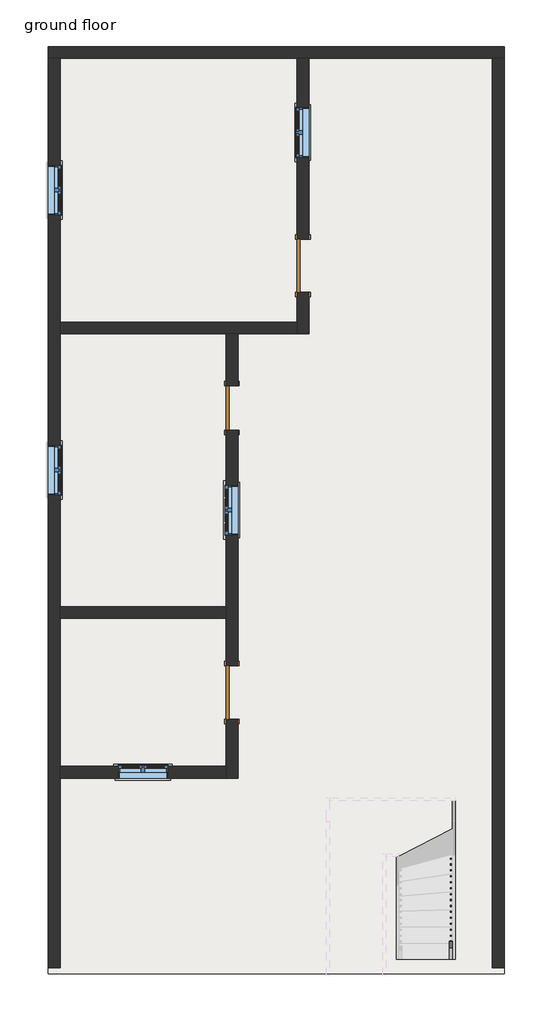
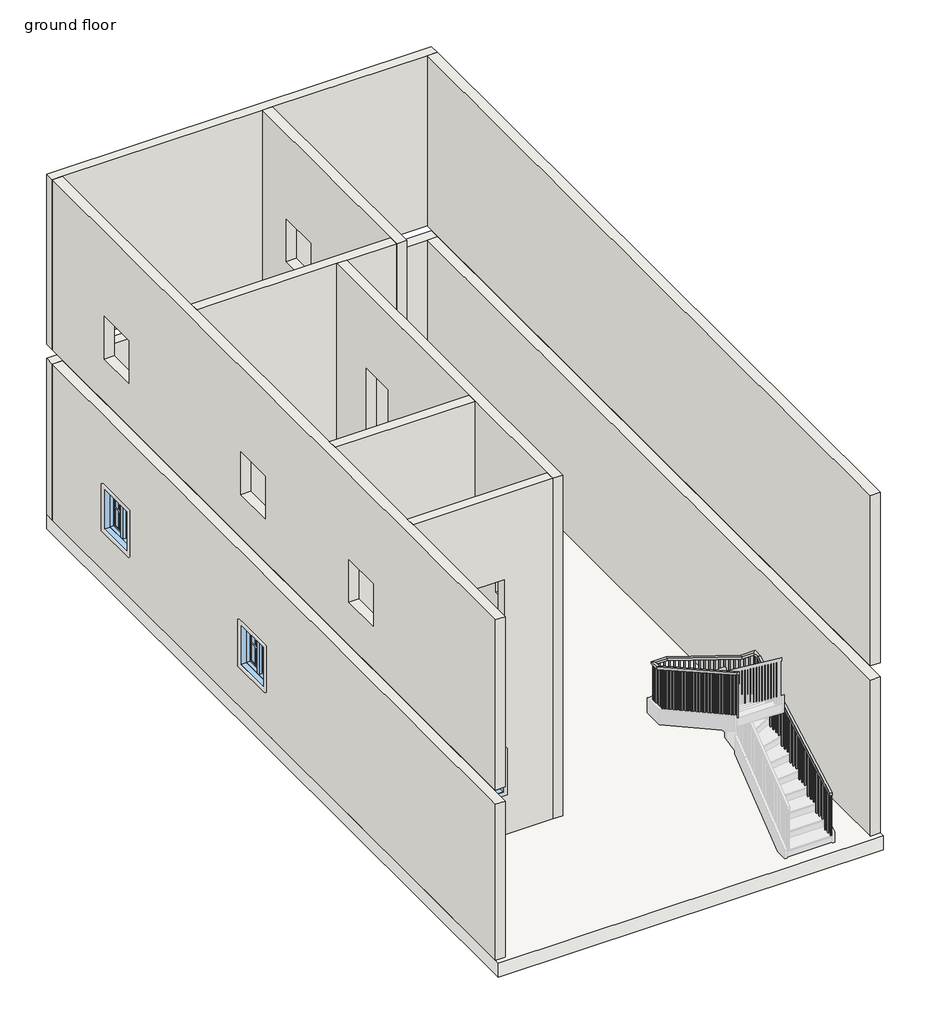
# One storey, part 1 of 2: 8 walls, 5 windows, 3 doors, 2 slabs, 1 railing.
"""IFC4 building model written with IfcOpenShell, lengths in millimetres."""

from ifc_helpers import new_model, si_unit, frame, origin, place, context, project, spatial, polyline, outline, extrude, faceted_brep, transform, mapped, element, save
from components import door_b6acaa4e, door_54dd4da4, door_719f80de, window_c29befe5, window_99681c7d

model = new_model("IFC4")

# Units and contexts
model_context = context("Model", 3, world=origin())
ifc_project = project(units=[si_unit("LENGTHUNIT", "METRE", prefix="MILLI")], contexts=[model_context])

# Site, building, storey
site = spatial("IfcSite", under=ifc_project)
building = spatial("IfcBuilding", under=site)
storey = spatial("IfcBuildingStorey", under=building, Name="ground floor", Elevation=1828.8)

# Doors
placement = place(None, origin())
door_shape = door_b6acaa4e(model_context)
element("IfcDoor", 1, ObjectType="Single-Flush : 30\" x 84\"", at=placement, inside=storey, context=model_context, shape_type="MappedRepresentation", body=[
    mapped(door_shape, transform((-12734.4887549, 9866.3027962, 1828.8), x_axis=(0.0, 1.0, 0.0), y_axis=(-1.0, 0.0, 0.0), z_axis=(0.0, 0.0, 1.0))),
])
door_2_shape = door_54dd4da4(model_context)
element("IfcDoor", 2, ObjectType="Single-Flush : 36\" x 84\"", at=placement, inside=storey, context=model_context, shape_type="MappedRepresentation", body=[
    mapped(door_2_shape, transform((-12734.4887549, 4989.5027962, 1828.8), x_axis=(0.0, 1.0, 0.0), y_axis=(-1.0, 0.0, 0.0), z_axis=(0.0, 0.0, 1.0))),
])
door_3_shape = door_719f80de(model_context)
element("IfcDoor", 3, ObjectType="Single-Flush : 36\" x 84\"", at=placement, inside=storey, context=model_context, shape_type="MappedRepresentation", body=[
    mapped(door_3_shape, transform((-11515.2887549, 12304.7027962, 1828.8), x_axis=(0.0, -1.0, 0.0), y_axis=(1.0, 0.0, 0.0), z_axis=(0.0, 0.0, 1.0))),
])

# Railing
element("IfcRailing", 4, ObjectType="Handrail - Rectangular", at=placement, inside=storey, context=model_context, shape_type="SolidModel", body=[
    faceted_brep([(-9000.6887549, 413.7711043, 2917.3714286), (-9000.6887549, 413.7711043, 2859.302637), (-8949.8887549, 413.7711043, 2859.302637), (-8949.8887549, 413.7711043, 2917.3714286), (-9000.6887549, 2949.2841703, 4321.4291136), (-9000.6887549, 2962.4104944, 4270.6291136), (-8949.8887549, 2962.4104944, 4270.6291136), (-8949.8887549, 2949.2841703, 4321.4291136), (-9252.9468652, 3084.5027962, 4270.6291136), (-9244.780431, 3084.5027962, 4321.4291136), (-10757.3244342, 3084.5027962, 4820.6326651), (-10765.4908683, 3084.5027962, 4769.8326651), (-9252.9468652, 3135.3027962, 4270.6291136), (-10765.4908683, 3135.3027962, 4769.8326651), (-9244.780431, 3135.3027962, 4321.4291136), (-10757.3244342, 3135.3027962, 4820.6326651), (-11007.2887549, 134.3711043, 6400.8), (-11058.0887549, 134.3711043, 6400.8), (-11058.0887549, 134.3711043, 6342.5372273), (-11007.2887549, 134.3711043, 6342.5372273), (-11007.2887549, 2934.7866859, 4769.8326651), (-11007.2887549, 2948.0751733, 4820.6326651), (-11058.0887549, 2934.7866859, 4769.8326651), (-11058.0887549, 2948.0751733, 4820.6326651), (-9000.6887549, 3084.5027962, 4321.4291136), (-9000.6887549, 3084.5027962, 4270.6291136), (-8949.8887549, 3135.3027962, 4270.6291136), (-8949.8887549, 3135.3027962, 4321.4291136), (-11007.2887549, 3084.5027962, 4820.6326651), (-11007.2887549, 3084.5027962, 4769.8326651), (-11058.0887549, 3135.3027962, 4769.8326651), (-11058.0887549, 3135.3027962, 4820.6326651)], [[[0, 1, 2, 3]], [[1, 0, 4, 5]], [[2, 1, 5, 6]], [[3, 2, 6, 7]], [[0, 3, 7, 4]], [[8, 9, 10, 11]], [[12, 8, 11, 13]], [[14, 12, 13, 15]], [[9, 14, 15, 10]], [[16, 17, 18, 19]], [[20, 21, 16, 19]], [[22, 20, 19, 18]], [[23, 22, 18, 17]], [[21, 23, 17, 16]], [[5, 4, 24, 25]], [[6, 5, 25, 26]], [[7, 6, 26, 27]], [[4, 7, 27, 24]], [[25, 24, 9, 8]], [[26, 25, 8, 12]], [[27, 26, 12, 14]], [[24, 27, 14, 9]], [[11, 10, 28, 29]], [[13, 11, 29, 30]], [[15, 13, 30, 31]], [[10, 15, 31, 28]], [[29, 28, 21, 20]], [[30, 29, 20, 22]], [[31, 30, 22, 23]], [[28, 31, 23, 21]]]),
    extrude(outline(polyline([(153.9777962, 6331.526171), (173.0277962, 6320.827751), (173.0277962, 5312.2285714), (153.9777962, 5312.2285714), (153.9777962, 6331.526171)])), frame((-11042.2137549, 0.0, 0.0), z_axis=(1.0, 0.0, 0.0), x_axis=(0.0, 1.0, 0.0)), (0.0, 0.0, 1.0), 19.05),
    extrude(outline(polyline([(255.5777962, 6274.4679313), (274.6277962, 6263.7695113), (274.6277962, 5312.2285714), (255.5777962, 5312.2285714), (255.5777962, 6274.4679313)])), frame((-11042.2137549, 0.0, 0.0), z_axis=(1.0, 0.0, 0.0), x_axis=(0.0, 1.0, 0.0)), (0.0, 0.0, 1.0), 19.05),
    extrude(outline(polyline([(357.1777962, 6217.4096916), (376.2277962, 6206.7112716), (376.2277962, 5312.2285714), (357.1777962, 5312.2285714), (357.1777962, 6217.4096916)])), frame((-11042.2137549, 0.0, 0.0), z_axis=(1.0, 0.0, 0.0), x_axis=(0.0, 1.0, 0.0)), (0.0, 0.0, 1.0), 19.05),
    extrude(outline(polyline([(458.7777962, 6160.3514519), (477.8277962, 6149.6530319), (477.8277962, 5138.0571429), (458.7777962, 5138.0571429), (458.7777962, 6160.3514519)])), frame((-11042.2137549, 0.0, 0.0), z_axis=(1.0, 0.0, 0.0), x_axis=(0.0, 1.0, 0.0)), (0.0, 0.0, 1.0), 19.05),
    extrude(outline(polyline([(560.3777962, 6103.2932122), (579.4277962, 6092.5947922), (579.4277962, 5138.0571429), (560.3777962, 5138.0571429), (560.3777962, 6103.2932122)])), frame((-11042.2137549, 0.0, 0.0), z_axis=(1.0, 0.0, 0.0), x_axis=(0.0, 1.0, 0.0)), (0.0, 0.0, 1.0), 19.05),
    extrude(outline(polyline([(661.9777962, 6046.2349725), (681.0277962, 6035.5365525), (681.0277962, 5138.0571429), (661.9777962, 5138.0571429), (661.9777962, 6046.2349725)])), frame((-11042.2137549, 0.0, 0.0), z_axis=(1.0, 0.0, 0.0), x_axis=(0.0, 1.0, 0.0)), (0.0, 0.0, 1.0), 19.05),
    extrude(outline(polyline([(763.5777962, 5989.1767328), (782.6277962, 5978.4783128), (782.6277962, 4963.8857143), (763.5777962, 4963.8857143), (763.5777962, 5989.1767328)])), frame((-11042.2137549, 0.0, 0.0), z_axis=(1.0, 0.0, 0.0), x_axis=(0.0, 1.0, 0.0)), (0.0, 0.0, 1.0), 19.05),
    extrude(outline(polyline([(865.1777962, 5932.1184931), (884.2277962, 5921.4200731), (884.2277962, 4963.8857143), (865.1777962, 4963.8857143), (865.1777962, 5932.1184931)])), frame((-11042.2137549, 0.0, 0.0), z_axis=(1.0, 0.0, 0.0), x_axis=(0.0, 1.0, 0.0)), (0.0, 0.0, 1.0), 19.05),
    extrude(outline(polyline([(966.7777962, 5875.0602534), (985.8277962, 5864.3618334), (985.8277962, 4963.8857143), (966.7777962, 4963.8857143), (966.7777962, 5875.0602534)])), frame((-11042.2137549, 0.0, 0.0), z_axis=(1.0, 0.0, 0.0), x_axis=(0.0, 1.0, 0.0)), (0.0, 0.0, 1.0), 19.05),
    extrude(outline(polyline([(1068.3777962, 5818.0020137), (1087.4277962, 5807.3035937), (1087.4277962, 4789.7142857), (1068.3777962, 4789.7142857), (1068.3777962, 5818.0020137)])), frame((-11042.2137549, 0.0, 0.0), z_axis=(1.0, 0.0, 0.0), x_axis=(0.0, 1.0, 0.0)), (0.0, 0.0, 1.0), 19.05),
    extrude(outline(polyline([(1169.9777962, 5760.943774), (1189.0277962, 5750.245354), (1189.0277962, 4789.7142857), (1169.9777962, 4789.7142857), (1169.9777962, 5760.943774)])), frame((-11042.2137549, 0.0, 0.0), z_axis=(1.0, 0.0, 0.0), x_axis=(0.0, 1.0, 0.0)), (0.0, 0.0, 1.0), 19.05),
    extrude(outline(polyline([(1271.5777962, 5703.8855343), (1290.6277962, 5693.1871143), (1290.6277962, 4615.5428571), (1271.5777962, 4615.5428571), (1271.5777962, 5703.8855343)])), frame((-11042.2137549, 0.0, 0.0), z_axis=(1.0, 0.0, 0.0), x_axis=(0.0, 1.0, 0.0)), (0.0, 0.0, 1.0), 19.05),
    extrude(outline(polyline([(1373.1777962, 5646.8272946), (1392.2277962, 5636.1288746), (1392.2277962, 4615.5428571), (1373.1777962, 4615.5428571), (1373.1777962, 5646.8272946)])), frame((-11042.2137549, 0.0, 0.0), z_axis=(1.0, 0.0, 0.0), x_axis=(0.0, 1.0, 0.0)), (0.0, 0.0, 1.0), 19.05),
    extrude(outline(polyline([(1474.7777962, 5589.6719878), (1493.8277962, 5579.1229201), (1493.8277962, 4615.5428571), (1474.7777962, 4615.5428571), (1474.7777962, 5589.6719878)])), frame((-11042.2137549, 0.0, 0.0), z_axis=(1.0, 0.0, 0.0), x_axis=(0.0, 1.0, 0.0)), (0.0, 0.0, 1.0), 19.05),
    extrude(outline(polyline([(1576.3777962, 5532.7108152), (1595.4277962, 5522.0123952), (1595.4277962, 4441.3714286), (1576.3777962, 4441.3714286), (1576.3777962, 5532.7108152)])), frame((-11042.2137549, 0.0, 0.0), z_axis=(1.0, 0.0, 0.0), x_axis=(0.0, 1.0, 0.0)), (0.0, 0.0, 1.0), 19.05),
    extrude(outline(polyline([(1677.9777962, 5475.6525755), (1697.0277962, 5464.9541555), (1697.0277962, 4441.3714286), (1677.9777962, 4441.3714286), (1677.9777962, 5475.6525755)])), frame((-11042.2137549, 0.0, 0.0), z_axis=(1.0, 0.0, 0.0), x_axis=(0.0, 1.0, 0.0)), (0.0, 0.0, 1.0), 19.05),
    extrude(outline(polyline([(1779.5777962, 5418.5943358), (1798.6277962, 5407.8959158), (1798.6277962, 4441.3714286), (1779.5777962, 4441.3714286), (1779.5777962, 5418.5943358)])), frame((-11042.2137549, 0.0, 0.0), z_axis=(1.0, 0.0, 0.0), x_axis=(0.0, 1.0, 0.0)), (0.0, 0.0, 1.0), 19.05),
    extrude(outline(polyline([(1881.1777962, 5361.536096), (1900.2277962, 5350.8376761), (1900.2277962, 4267.2), (1881.1777962, 4267.2), (1881.1777962, 5361.536096)])), frame((-11042.2137549, 0.0, 0.0), z_axis=(1.0, 0.0, 0.0), x_axis=(0.0, 1.0, 0.0)), (0.0, 0.0, 1.0), 19.05),
    extrude(outline(polyline([(1982.7777962, 5304.4778563), (2001.8277962, 5293.7794364), (2001.8277962, 4267.2), (1982.7777962, 4267.2), (1982.7777962, 5304.4778563)])), frame((-11042.2137549, 0.0, 0.0), z_axis=(1.0, 0.0, 0.0), x_axis=(0.0, 1.0, 0.0)), (0.0, 0.0, 1.0), 19.05),
    extrude(outline(polyline([(2084.3777962, 5247.4196166), (2103.4277962, 5236.7211967), (2103.4277962, 4267.2), (2084.3777962, 4267.2), (2084.3777962, 5247.4196166)])), frame((-11042.2137549, 0.0, 0.0), z_axis=(1.0, 0.0, 0.0), x_axis=(0.0, 1.0, 0.0)), (0.0, 0.0, 1.0), 19.05),
    extrude(outline(polyline([(2185.9777962, 5190.3613769), (2205.0277962, 5179.662957), (2205.0277962, 4267.2), (2185.9777962, 4267.2), (2185.9777962, 5190.3613769)])), frame((-11042.2137549, 0.0, 0.0), z_axis=(1.0, 0.0, 0.0), x_axis=(0.0, 1.0, 0.0)), (0.0, 0.0, 1.0), 19.05),
    extrude(outline(polyline([(2287.5777962, 5133.3031372), (2306.6277962, 5122.6047173), (2306.6277962, 4093.0285714), (2287.5777962, 4093.0285714), (2287.5777962, 5133.3031372)])), frame((-11042.2137549, 0.0, 0.0), z_axis=(1.0, 0.0, 0.0), x_axis=(0.0, 1.0, 0.0)), (0.0, 0.0, 1.0), 19.05),
    extrude(outline(polyline([(2389.1777962, 5076.2448975), (2408.2277962, 5065.5464776), (2408.2277962, 4093.0285714), (2389.1777962, 4093.0285714), (2389.1777962, 5076.2448975)])), frame((-11042.2137549, 0.0, 0.0), z_axis=(1.0, 0.0, 0.0), x_axis=(0.0, 1.0, 0.0)), (0.0, 0.0, 1.0), 19.05),
    extrude(outline(polyline([(2490.7777962, 5019.1866578), (2509.8277962, 5008.4882379), (2509.8277962, 4093.0285714), (2490.7777962, 4093.0285714), (2490.7777962, 5019.1866578)])), frame((-11042.2137549, 0.0, 0.0), z_axis=(1.0, 0.0, 0.0), x_axis=(0.0, 1.0, 0.0)), (0.0, 0.0, 1.0), 19.05),
    extrude(outline(polyline([(2592.3777962, 4962.1284181), (2611.4277962, 4951.4299982), (2611.4277962, 4093.0285714), (2592.3777962, 4093.0285714), (2592.3777962, 4962.1284181)])), frame((-11042.2137549, 0.0, 0.0), z_axis=(1.0, 0.0, 0.0), x_axis=(0.0, 1.0, 0.0)), (0.0, 0.0, 1.0), 19.05),
    extrude(outline(polyline([(2693.9777962, 4905.0701784), (2713.0277962, 4894.3717585), (2713.0277962, 3918.8571429), (2693.9777962, 3918.8571429), (2693.9777962, 4905.0701784)])), frame((-11042.2137549, 0.0, 0.0), z_axis=(1.0, 0.0, 0.0), x_axis=(0.0, 1.0, 0.0)), (0.0, 0.0, 1.0), 19.05),
    extrude(outline(polyline([(2795.5777962, 4848.0119387), (2814.6277962, 4837.3135188), (2814.6277962, 3918.8571429), (2795.5777962, 3918.8571429), (2795.5777962, 4848.0119387)])), frame((-11042.2137549, 0.0, 0.0), z_axis=(1.0, 0.0, 0.0), x_axis=(0.0, 1.0, 0.0)), (0.0, 0.0, 1.0), 19.05),
    extrude(outline(polyline([(2897.1777962, 4790.953699), (2916.2277962, 4780.2552791), (2916.2277962, 3918.8571429), (2897.1777962, 3918.8571429), (2897.1777962, 4790.953699)])), frame((-11042.2137549, 0.0, 0.0), z_axis=(1.0, 0.0, 0.0), x_axis=(0.0, 1.0, 0.0)), (0.0, 0.0, 1.0), 19.05),
    extrude(outline(polyline([(-11042.2137549, 3017.8277962), (-11023.1637549, 3017.8277962), (-11023.1637549, 2998.7777962), (-11042.2137549, 2998.7777962), (-11042.2137549, 3017.8277962)])), frame((0.0, 0.0, 3918.8571429), z_axis=(0.0, 0.0, 1.0), x_axis=(1.0, 0.0, 0.0)), (0.0, 0.0, 1.0), 850.9755223),
    extrude(outline(polyline([(-10997.7637549, 3119.4277962), (-10997.7637549, 3100.3777962), (-11016.8137549, 3100.3777962), (-11016.8137549, 3119.4277962), (-10997.7637549, 3119.4277962)])), frame((0.0, 0.0, 3918.8571429), z_axis=(0.0, 0.0, 1.0), x_axis=(1.0, 0.0, 0.0)), (0.0, 0.0, 1.0), 850.9755223),
    extrude(outline(polyline([(-10896.1637549, 3119.4277962), (-10896.1637549, 3100.3777962), (-10915.2137549, 3100.3777962), (-10915.2137549, 3119.4277962), (-10896.1637549, 3119.4277962)])), frame((0.0, 0.0, 3918.8571429), z_axis=(0.0, 0.0, 1.0), x_axis=(1.0, 0.0, 0.0)), (0.0, 0.0, 1.0), 850.9755223),
    extrude(outline(polyline([(-10794.5637549, 3119.4277962), (-10794.5637549, 3100.3777962), (-10813.6137549, 3100.3777962), (-10813.6137549, 3119.4277962), (-10794.5637549, 3119.4277962)])), frame((0.0, 0.0, 3918.8571429), z_axis=(0.0, 0.0, 1.0), x_axis=(1.0, 0.0, 0.0)), (0.0, 0.0, 1.0), 850.9755223),
    extrude(outline(polyline([(4745.8956474, -10692.9637549), (4752.1829538, -10712.0137549), (3744.6857143, -10712.0137549), (3744.6857143, -10692.9637549), (4745.8956474, -10692.9637549)])), frame((0.0, 3100.3777962, 0.0), z_axis=(0.0, 1.0, 0.0), x_axis=(0.0, 0.0, 1.0)), (0.0, 0.0, 1.0), 19.05),
    extrude(outline(polyline([(4712.3633464, -10591.3637549), (4718.6506528, -10610.4137549), (3744.6857143, -10610.4137549), (3744.6857143, -10591.3637549), (4712.3633464, -10591.3637549)])), frame((0.0, 3100.3777962, 0.0), z_axis=(0.0, 1.0, 0.0), x_axis=(0.0, 0.0, 1.0)), (0.0, 0.0, 1.0), 19.05),
    extrude(outline(polyline([(4678.8310453, -10489.7637549), (4685.1183518, -10508.8137549), (3744.6857143, -10508.8137549), (3744.6857143, -10489.7637549), (4678.8310453, -10489.7637549)])), frame((0.0, 3100.3777962, 0.0), z_axis=(0.0, 1.0, 0.0), x_axis=(0.0, 0.0, 1.0)), (0.0, 0.0, 1.0), 19.05),
    extrude(outline(polyline([(4645.2987443, -10388.1637549), (4651.5860507, -10407.2137549), (3744.6857143, -10407.2137549), (3744.6857143, -10388.1637549), (4645.2987443, -10388.1637549)])), frame((0.0, 3100.3777962, 0.0), z_axis=(0.0, 1.0, 0.0), x_axis=(0.0, 0.0, 1.0)), (0.0, 0.0, 1.0), 19.05),
    extrude(outline(polyline([(4611.7664433, -10286.5637549), (4618.0537497, -10305.6137549), (3744.6857143, -10305.6137549), (3744.6857143, -10286.5637549), (4611.7664433, -10286.5637549)])), frame((0.0, 3100.3777962, 0.0), z_axis=(0.0, 1.0, 0.0), x_axis=(0.0, 0.0, 1.0)), (0.0, 0.0, 1.0), 19.05),
    extrude(outline(polyline([(4578.2341422, -10184.9637549), (4584.5214487, -10204.0137549), (3570.5142857, -10204.0137549), (3570.5142857, -10184.9637549), (4578.2341422, -10184.9637549)])), frame((0.0, 3100.3777962, 0.0), z_axis=(0.0, 1.0, 0.0), x_axis=(0.0, 0.0, 1.0)), (0.0, 0.0, 1.0), 19.05),
    extrude(outline(polyline([(4544.7018412, -10083.3637549), (4550.9891476, -10102.4137549), (3570.5142857, -10102.4137549), (3570.5142857, -10083.3637549), (4544.7018412, -10083.3637549)])), frame((0.0, 3100.3777962, 0.0), z_axis=(0.0, 1.0, 0.0), x_axis=(0.0, 0.0, 1.0)), (0.0, 0.0, 1.0), 19.05),
    extrude(outline(polyline([(4511.1695402, -9981.7637549), (4517.4568466, -10000.8137549), (3570.5142857, -10000.8137549), (3570.5142857, -9981.7637549), (4511.1695402, -9981.7637549)])), frame((0.0, 3100.3777962, 0.0), z_axis=(0.0, 1.0, 0.0), x_axis=(0.0, 0.0, 1.0)), (0.0, 0.0, 1.0), 19.05),
    extrude(outline(polyline([(4477.6372391, -9880.1637549), (4483.9245456, -9899.2137549), (3570.5142857, -9899.2137549), (3570.5142857, -9880.1637549), (4477.6372391, -9880.1637549)])), frame((0.0, 3100.3777962, 0.0), z_axis=(0.0, 1.0, 0.0), x_axis=(0.0, 0.0, 1.0)), (0.0, 0.0, 1.0), 19.05),
    extrude(outline(polyline([(4444.1049381, -9778.5637549), (4450.3922445, -9797.6137549), (3570.5142857, -9797.6137549), (3570.5142857, -9778.5637549), (4444.1049381, -9778.5637549)])), frame((0.0, 3100.3777962, 0.0), z_axis=(0.0, 1.0, 0.0), x_axis=(0.0, 0.0, 1.0)), (0.0, 0.0, 1.0), 19.05),
    extrude(outline(polyline([(4410.5726371, -9676.9637549), (4416.8599435, -9696.0137549), (3396.3428571, -9696.0137549), (3396.3428571, -9676.9637549), (4410.5726371, -9676.9637549)])), frame((0.0, 3100.3777962, 0.0), z_axis=(0.0, 1.0, 0.0), x_axis=(0.0, 0.0, 1.0)), (0.0, 0.0, 1.0), 19.05),
    extrude(outline(polyline([(4377.040336, -9575.3637549), (4383.3276425, -9594.4137549), (3396.3428571, -9594.4137549), (3396.3428571, -9575.3637549), (4377.040336, -9575.3637549)])), frame((0.0, 3100.3777962, 0.0), z_axis=(0.0, 1.0, 0.0), x_axis=(0.0, 0.0, 1.0)), (0.0, 0.0, 1.0), 19.05),
    extrude(outline(polyline([(4343.508035, -9473.7637549), (4349.7953414, -9492.8137549), (3396.3428571, -9492.8137549), (3396.3428571, -9473.7637549), (4343.508035, -9473.7637549)])), frame((0.0, 3100.3777962, 0.0), z_axis=(0.0, 1.0, 0.0), x_axis=(0.0, 0.0, 1.0)), (0.0, 0.0, 1.0), 19.05),
    extrude(outline(polyline([(4309.975734, -9372.1637549), (4316.2630404, -9391.2137549), (3396.3428571, -9391.2137549), (3396.3428571, -9372.1637549), (4309.975734, -9372.1637549)])), frame((0.0, 3100.3777962, 0.0), z_axis=(0.0, 1.0, 0.0), x_axis=(0.0, 0.0, 1.0)), (0.0, 0.0, 1.0), 19.05),
    extrude(outline(polyline([(4276.4434329, -9270.5637549), (4282.7307394, -9289.6137549), (3396.3428571, -9289.6137549), (3396.3428571, -9270.5637549), (4276.4434329, -9270.5637549)])), frame((0.0, 3100.3777962, 0.0), z_axis=(0.0, 1.0, 0.0), x_axis=(0.0, 0.0, 1.0)), (0.0, 0.0, 1.0), 19.05),
    extrude(outline(polyline([(-9168.9637549, 3119.4277962), (-9168.9637549, 3100.3777962), (-9188.0137549, 3100.3777962), (-9188.0137549, 3119.4277962), (-9168.9637549, 3119.4277962)])), frame((0.0, 0.0, 3222.1714286), z_axis=(0.0, 0.0, 1.0), x_axis=(1.0, 0.0, 0.0)), (0.0, 0.0, 1.0), 1048.457685),
    extrude(outline(polyline([(-9067.3637549, 3119.4277962), (-9067.3637549, 3100.3777962), (-9086.4137549, 3100.3777962), (-9086.4137549, 3119.4277962), (-9067.3637549, 3119.4277962)])), frame((0.0, 0.0, 3222.1714286), z_axis=(0.0, 0.0, 1.0), x_axis=(1.0, 0.0, 0.0)), (0.0, 0.0, 1.0), 1048.457685),
    extrude(outline(polyline([(-8965.7637549, 3045.8461043), (-8984.8137549, 3045.8461043), (-8984.8137549, 3064.8961043), (-8965.7637549, 3064.8961043), (-8965.7637549, 3045.8461043)])), frame((0.0, 0.0, 3222.1714286), z_axis=(0.0, 0.0, 1.0), x_axis=(1.0, 0.0, 0.0)), (0.0, 0.0, 1.0), 1048.457685),
    extrude(outline(polyline([(-8965.7637549, 2944.2461043), (-8984.8137549, 2944.2461043), (-8984.8137549, 2963.2961043), (-8965.7637549, 2963.2961043), (-8965.7637549, 2944.2461043)])), frame((0.0, 0.0, 3222.1714286), z_axis=(0.0, 0.0, 1.0), x_axis=(1.0, 0.0, 0.0)), (0.0, 0.0, 1.0), 1048.457685),
    extrude(outline(polyline([(2842.6461043, 4204.3087643), (2861.6961043, 4214.8578319), (2861.6961043, 3222.1714286), (2842.6461043, 3222.1714286), (2842.6461043, 4204.3087643)])), frame((-8984.8137549, 0.0, 0.0), z_axis=(1.0, 0.0, 0.0), x_axis=(0.0, 1.0, 0.0)), (0.0, 0.0, 1.0), 19.05),
    extrude(outline(polyline([(2741.0461043, 4148.04707), (2760.0961043, 4158.5961377), (2760.0961043, 3222.1714286), (2741.0461043, 3222.1714286), (2741.0461043, 4148.04707)])), frame((-8984.8137549, 0.0, 0.0), z_axis=(1.0, 0.0, 0.0), x_axis=(0.0, 1.0, 0.0)), (0.0, 0.0, 1.0), 19.05),
    extrude(outline(polyline([(2639.4461043, 4091.7853758), (2658.4961043, 4102.3344435), (2658.4961043, 3222.1714286), (2639.4461043, 3222.1714286), (2639.4461043, 4091.7853758)])), frame((-8984.8137549, 0.0, 0.0), z_axis=(1.0, 0.0, 0.0), x_axis=(0.0, 1.0, 0.0)), (0.0, 0.0, 1.0), 19.05),
    extrude(outline(polyline([(2537.8461043, 4035.5236816), (2556.8961043, 4046.0727493), (2556.8961043, 3048.0), (2537.8461043, 3048.0), (2537.8461043, 4035.5236816)])), frame((-8984.8137549, 0.0, 0.0), z_axis=(1.0, 0.0, 0.0), x_axis=(0.0, 1.0, 0.0)), (0.0, 0.0, 1.0), 19.05),
    extrude(outline(polyline([(2436.2461043, 3979.2619874), (2455.2961043, 3989.8110551), (2455.2961043, 3048.0), (2436.2461043, 3048.0), (2436.2461043, 3979.2619874)])), frame((-8984.8137549, 0.0, 0.0), z_axis=(1.0, 0.0, 0.0), x_axis=(0.0, 1.0, 0.0)), (0.0, 0.0, 1.0), 19.05),
    extrude(outline(polyline([(2334.6461043, 3923.0002932), (2353.6961043, 3933.5493609), (2353.6961043, 3048.0), (2334.6461043, 3048.0), (2334.6461043, 3923.0002932)])), frame((-8984.8137549, 0.0, 0.0), z_axis=(1.0, 0.0, 0.0), x_axis=(0.0, 1.0, 0.0)), (0.0, 0.0, 1.0), 19.05),
    extrude(outline(polyline([(2233.0461043, 3866.738599), (2252.0961043, 3877.2876666), (2252.0961043, 3048.0), (2233.0461043, 3048.0), (2233.0461043, 3866.738599)])), frame((-8984.8137549, 0.0, 0.0), z_axis=(1.0, 0.0, 0.0), x_axis=(0.0, 1.0, 0.0)), (0.0, 0.0, 1.0), 19.05),
    extrude(outline(polyline([(2131.4461043, 3810.4769048), (2150.4961043, 3821.0259724), (2150.4961043, 2873.8285714), (2131.4461043, 2873.8285714), (2131.4461043, 3810.4769048)])), frame((-8984.8137549, 0.0, 0.0), z_axis=(1.0, 0.0, 0.0), x_axis=(0.0, 1.0, 0.0)), (0.0, 0.0, 1.0), 19.05),
    extrude(outline(polyline([(2029.8461043, 3754.2152105), (2048.8961043, 3764.7642782), (2048.8961043, 2873.8285714), (2029.8461043, 2873.8285714), (2029.8461043, 3754.2152105)])), frame((-8984.8137549, 0.0, 0.0), z_axis=(1.0, 0.0, 0.0), x_axis=(0.0, 1.0, 0.0)), (0.0, 0.0, 1.0), 19.05),
    extrude(outline(polyline([(1928.2461043, 3697.9535163), (1947.2961043, 3708.502584), (1947.2961043, 2873.8285714), (1928.2461043, 2873.8285714), (1928.2461043, 3697.9535163)])), frame((-8984.8137549, 0.0, 0.0), z_axis=(1.0, 0.0, 0.0), x_axis=(0.0, 1.0, 0.0)), (0.0, 0.0, 1.0), 19.05),
    extrude(outline(polyline([(1826.6461043, 3641.6918221), (1845.6961043, 3652.2408898), (1845.6961043, 2699.6571429), (1826.6461043, 2699.6571429), (1826.6461043, 3641.6918221)])), frame((-8984.8137549, 0.0, 0.0), z_axis=(1.0, 0.0, 0.0), x_axis=(0.0, 1.0, 0.0)), (0.0, 0.0, 1.0), 19.05),
    extrude(outline(polyline([(1725.0461043, 3585.4301279), (1744.0961043, 3595.9791956), (1744.0961043, 2699.6571429), (1725.0461043, 2699.6571429), (1725.0461043, 3585.4301279)])), frame((-8984.8137549, 0.0, 0.0), z_axis=(1.0, 0.0, 0.0), x_axis=(0.0, 1.0, 0.0)), (0.0, 0.0, 1.0), 19.05),
    extrude(outline(polyline([(1623.4461043, 3529.1684337), (1642.4961043, 3539.7175014), (1642.4961043, 2699.6571429), (1623.4461043, 2699.6571429), (1623.4461043, 3529.1684337)])), frame((-8984.8137549, 0.0, 0.0), z_axis=(1.0, 0.0, 0.0), x_axis=(0.0, 1.0, 0.0)), (0.0, 0.0, 1.0), 19.05),
    extrude(outline(polyline([(1521.8461043, 3472.9067395), (1540.8961043, 3483.4558071), (1540.8961043, 2525.4857143), (1521.8461043, 2525.4857143), (1521.8461043, 3472.9067395)])), frame((-8984.8137549, 0.0, 0.0), z_axis=(1.0, 0.0, 0.0), x_axis=(0.0, 1.0, 0.0)), (0.0, 0.0, 1.0), 19.05),
    extrude(outline(polyline([(1420.2461043, 3416.6450453), (1439.2961043, 3427.1941129), (1439.2961043, 2525.4857143), (1420.2461043, 2525.4857143), (1420.2461043, 3416.6450453)])), frame((-8984.8137549, 0.0, 0.0), z_axis=(1.0, 0.0, 0.0), x_axis=(0.0, 1.0, 0.0)), (0.0, 0.0, 1.0), 19.05),
    extrude(outline(polyline([(1318.6461043, 3360.3833511), (1337.6961043, 3370.9324187), (1337.6961043, 2525.4857143), (1318.6461043, 2525.4857143), (1318.6461043, 3360.3833511)])), frame((-8984.8137549, 0.0, 0.0), z_axis=(1.0, 0.0, 0.0), x_axis=(0.0, 1.0, 0.0)), (0.0, 0.0, 1.0), 19.05),
    extrude(outline(polyline([(1217.0461043, 3304.1216568), (1236.0961043, 3314.6707245), (1236.0961043, 2351.3142857), (1217.0461043, 2351.3142857), (1217.0461043, 3304.1216568)])), frame((-8984.8137549, 0.0, 0.0), z_axis=(1.0, 0.0, 0.0), x_axis=(0.0, 1.0, 0.0)), (0.0, 0.0, 1.0), 19.05),
    extrude(outline(polyline([(1115.4461043, 3247.8599626), (1134.4961043, 3258.4090303), (1134.4961043, 2351.3142857), (1115.4461043, 2351.3142857), (1115.4461043, 3247.8599626)])), frame((-8984.8137549, 0.0, 0.0), z_axis=(1.0, 0.0, 0.0), x_axis=(0.0, 1.0, 0.0)), (0.0, 0.0, 1.0), 19.05),
    extrude(outline(polyline([(1013.8461043, 3191.5982684), (1032.8961043, 3202.1473361), (1032.8961043, 2351.3142857), (1013.8461043, 2351.3142857), (1013.8461043, 3191.5982684)])), frame((-8984.8137549, 0.0, 0.0), z_axis=(1.0, 0.0, 0.0), x_axis=(0.0, 1.0, 0.0)), (0.0, 0.0, 1.0), 19.05),
    extrude(outline(polyline([(912.2461043, 3135.3365742), (931.2961043, 3145.8856419), (931.2961043, 2177.1428571), (912.2461043, 2177.1428571), (912.2461043, 3135.3365742)])), frame((-8984.8137549, 0.0, 0.0), z_axis=(1.0, 0.0, 0.0), x_axis=(0.0, 1.0, 0.0)), (0.0, 0.0, 1.0), 19.05),
    extrude(outline(polyline([(810.6461043, 3079.07488), (829.6961043, 3089.6239476), (829.6961043, 2177.1428571), (810.6461043, 2177.1428571), (810.6461043, 3079.07488)])), frame((-8984.8137549, 0.0, 0.0), z_axis=(1.0, 0.0, 0.0), x_axis=(0.0, 1.0, 0.0)), (0.0, 0.0, 1.0), 19.05),
    extrude(outline(polyline([(709.0461043, 3022.8131858), (728.0961043, 3033.3622534), (728.0961043, 2177.1428571), (709.0461043, 2177.1428571), (709.0461043, 3022.8131858)])), frame((-8984.8137549, 0.0, 0.0), z_axis=(1.0, 0.0, 0.0), x_axis=(0.0, 1.0, 0.0)), (0.0, 0.0, 1.0), 19.05),
    extrude(outline(polyline([(607.4461043, 2966.5514916), (626.4961043, 2977.1005592), (626.4961043, 2002.9714286), (607.4461043, 2002.9714286), (607.4461043, 2966.5514916)])), frame((-8984.8137549, 0.0, 0.0), z_axis=(1.0, 0.0, 0.0), x_axis=(0.0, 1.0, 0.0)), (0.0, 0.0, 1.0), 19.05),
    extrude(outline(polyline([(505.8461043, 2910.2897973), (524.8961043, 2920.838865), (524.8961043, 2002.9714286), (505.8461043, 2002.9714286), (505.8461043, 2910.2897973)])), frame((-8984.8137549, 0.0, 0.0), z_axis=(1.0, 0.0, 0.0), x_axis=(0.0, 1.0, 0.0)), (0.0, 0.0, 1.0), 19.05),
    extrude(outline(polyline([(-11023.1637549, 3119.4277962), (-11023.1637549, 3100.3777962), (-11042.2137549, 3100.3777962), (-11042.2137549, 3119.4277962), (-11023.1637549, 3119.4277962)])), frame((0.0, 0.0, 3918.8571429), z_axis=(0.0, 0.0, 1.0), x_axis=(1.0, 0.0, 0.0)), (0.0, 0.0, 1.0), 850.9755223),
    extrude(outline(polyline([(-8965.7637549, 3100.3777962), (-8984.8137549, 3100.3777962), (-8984.8137549, 3119.4277962), (-8965.7637549, 3119.4277962), (-8965.7637549, 3100.3777962)])), frame((0.0, 0.0, 3222.1714286), z_axis=(0.0, 0.0, 1.0), x_axis=(1.0, 0.0, 0.0)), (0.0, 0.0, 1.0), 1048.457685),
    extrude(outline(polyline([(134.3711043, 6342.5372273), (153.4211043, 6331.8388074), (153.4211043, 5312.2285714), (134.3711043, 5312.2285714), (134.3711043, 6342.5372273)])), frame((-11042.2137549, 0.0, 0.0), z_axis=(1.0, 0.0, 0.0), x_axis=(0.0, 1.0, 0.0)), (0.0, 0.0, 1.0), 19.05),
    extrude(outline(polyline([(413.7711043, 2859.302637), (432.8211043, 2869.8517046), (432.8211043, 2002.9714286), (413.7711043, 2002.9714286), (413.7711043, 2859.302637)])), frame((-8984.8137549, 0.0, 0.0), z_axis=(1.0, 0.0, 0.0), x_axis=(0.0, 1.0, 0.0)), (0.0, 0.0, 1.0), 19.05),
])

# Slabs
element("IfcSlab", 5, ObjectType="Generic - 12\"", at=placement, inside=storey, context=model_context, shape_type="SweptSolid", body=[
    extrude(outline(polyline([(-8060.8887549, 16063.9027962), (-8060.8887549, 163.5027962), (-15884.0887549, 163.5027962), (-15884.0887549, 16063.9027962), (-8060.8887549, 16063.9027962)])), frame((0.0, 0.0, 1524.0), z_axis=(0.0, 0.0, 1.0), x_axis=(1.0, 0.0, 0.0)), (0.0, 0.0, 1.0), 304.8),
])
element("IfcSlab", 6, ObjectType="Generic - 12\"", at=placement, inside=storey, context=model_context, shape_type="SweptSolid", body=[
    extrude(outline(polyline([(-8060.8887549, 16063.9027962), (-8060.8887549, 163.5027962), (-15884.0887549, 163.5027962), (-15884.0887549, 16063.9027962), (-8060.8887549, 16063.9027962)])), frame((0.0, 0.0, 1524.0), z_axis=(0.0, 0.0, 1.0), x_axis=(1.0, 0.0, 0.0)), (0.0, 0.0, 1.0), 304.8),
])

# Walls
element("IfcWall", 7, ObjectType="Generic - 8\"", at=placement, inside=storey, context=model_context, shape_type="SweptSolid", body=[
    extrude(outline(polyline([(-8264.0887549, 265.1027962), (-8264.0887549, 15860.7027962), (-8060.8887549, 15860.7027962), (-8060.8887549, 265.1027962), (-8264.0887549, 265.1027962)])), frame((0.0, 0.0, 1828.8), z_axis=(0.0, 0.0, 1.0), x_axis=(1.0, 0.0, 0.0)), (0.0, 0.0, 1.0), 3352.8),
    extrude(outline(polyline([(-8264.0887549, 265.1027962), (-8264.0887549, 15860.7027962), (-8060.8887549, 15860.7027962), (-8060.8887549, 265.1027962), (-8264.0887549, 265.1027962)])), frame((0.0, 0.0, 5486.4), z_axis=(0.0, 0.0, 1.0), x_axis=(1.0, 0.0, 0.0)), (0.0, 0.0, 1.0), 3657.6),
])
element("IfcWall", 8, ObjectType="Generic - 8\"", at=placement, inside=storey, context=model_context, shape_type="Brep", body=[
    faceted_brep([(-15884.0887549, 15860.7027962, 1828.8), (-15884.0887549, 265.1027962, 1828.8), (-15884.0887549, 265.1027962, 5181.6), (-15884.0887549, 15860.7027962, 5181.6), (-15884.0887549, 13168.3027962, 3657.6), (-15884.0887549, 13168.3027962, 2743.2), (-15884.0887549, 14031.9027962, 2743.2), (-15884.0887549, 14031.9027962, 3657.6), (-15884.0887549, 8367.7027962, 3657.6), (-15884.0887549, 8367.7027962, 2743.2), (-15884.0887549, 9231.3027962, 2743.2), (-15884.0887549, 9231.3027962, 3657.6), (-15680.8887549, 265.1027962, 1828.8), (-15680.8887549, 3516.3027962, 1828.8), (-15680.8887549, 3719.5027962, 1828.8), (-15680.8887549, 6259.5027962, 1828.8), (-15680.8887549, 6462.7027962, 1828.8), (-15680.8887549, 11136.3027962, 1828.8), (-15680.8887549, 11339.5027962, 1828.8), (-15680.8887549, 15860.7027962, 1828.8), (-15680.8887549, 15860.7027962, 5181.6), (-15680.8887549, 265.1027962, 5181.6), (-15680.8887549, 13168.3027962, 2743.2), (-15680.8887549, 13168.3027962, 3657.6), (-15680.8887549, 14031.9027962, 3657.6), (-15680.8887549, 14031.9027962, 2743.2), (-15680.8887549, 8367.7027962, 2743.2), (-15680.8887549, 8367.7027962, 3657.6), (-15680.8887549, 9231.3027962, 3657.6), (-15680.8887549, 9231.3027962, 2743.2)], [[[0, 1, 2, 3], [4, 5, 6, 7], [8, 9, 10, 11]], [[12, 13, 14, 15, 16, 17, 18, 19, 20, 21], [22, 23, 24, 25], [26, 27, 28, 29]], [[1, 0, 19, 18, 17, 16, 15, 14, 13, 12]], [[1, 12, 21, 2]], [[19, 0, 3, 20]], [[3, 2, 21, 20]], [[5, 4, 23, 22]], [[6, 5, 22, 25]], [[7, 6, 25, 24]], [[4, 7, 24, 23]], [[9, 8, 27, 26]], [[10, 9, 26, 29]], [[11, 10, 29, 28]], [[8, 11, 28, 27]]]),
    faceted_brep([(-15884.0887549, 265.1027962, 9144.0), (-15884.0887549, 15860.7027962, 9144.0), (-15884.0887549, 15860.7027962, 5486.4), (-15884.0887549, 265.1027962, 5486.4), (-15884.0887549, 13168.3027962, 7315.2), (-15884.0887549, 13168.3027962, 6400.8), (-15884.0887549, 14031.9027962, 6400.8), (-15884.0887549, 14031.9027962, 7315.2), (-15884.0887549, 8367.7027962, 7315.2), (-15884.0887549, 8367.7027962, 6400.8), (-15884.0887549, 9231.3027962, 6400.8), (-15884.0887549, 9231.3027962, 7315.2), (-15884.0887549, 4557.7027962, 7315.2), (-15884.0887549, 4557.7027962, 6400.8), (-15884.0887549, 5421.3027962, 6400.8), (-15884.0887549, 5421.3027962, 7315.2), (-15680.8887549, 15860.7027962, 9144.0), (-15680.8887549, 11339.5027962, 9144.0), (-15680.8887549, 11136.3027962, 9144.0), (-15680.8887549, 6462.7027962, 9144.0), (-15680.8887549, 6259.5027962, 9144.0), (-15680.8887549, 3719.5027962, 9144.0), (-15680.8887549, 3516.3027962, 9144.0), (-15680.8887549, 265.1027962, 9144.0), (-15680.8887549, 265.1027962, 5486.4), (-15680.8887549, 15860.7027962, 5486.4), (-15680.8887549, 13168.3027962, 6400.8), (-15680.8887549, 13168.3027962, 7315.2), (-15680.8887549, 14031.9027962, 7315.2), (-15680.8887549, 14031.9027962, 6400.8), (-15680.8887549, 8367.7027962, 6400.8), (-15680.8887549, 8367.7027962, 7315.2), (-15680.8887549, 9231.3027962, 7315.2), (-15680.8887549, 9231.3027962, 6400.8), (-15680.8887549, 4557.7027962, 6400.8), (-15680.8887549, 4557.7027962, 7315.2), (-15680.8887549, 5421.3027962, 7315.2), (-15680.8887549, 5421.3027962, 6400.8)], [[[0, 1, 2, 3], [4, 5, 6, 7], [8, 9, 10, 11], [12, 13, 14, 15]], [[16, 17, 18, 19, 20, 21, 22, 23, 24, 25], [26, 27, 28, 29], [30, 31, 32, 33], [34, 35, 36, 37]], [[23, 0, 3, 24]], [[1, 0, 23, 22, 21, 20, 19, 18, 17, 16]], [[1, 16, 25, 2]], [[3, 2, 25, 24]], [[5, 4, 27, 26]], [[6, 5, 26, 29]], [[7, 6, 29, 28]], [[4, 7, 28, 27]], [[9, 8, 31, 30]], [[10, 9, 30, 33]], [[11, 10, 33, 32]], [[8, 11, 32, 31]], [[13, 12, 35, 34]], [[14, 13, 34, 37]], [[15, 14, 37, 36]], [[12, 15, 36, 35]]]),
])
element("IfcWall", 9, ObjectType="Generic - 8\"", at=placement, inside=storey, context=model_context, shape_type="Brep", body=[
    faceted_brep([(-11616.8887549, 11847.5027962, 3962.4), (-11616.8887549, 11847.5027962, 1828.8), (-11616.8887549, 11339.5027962, 1828.8), (-11616.8887549, 11136.3027962, 1828.8), (-11616.8887549, 11136.3027962, 9144.0), (-11616.8887549, 11339.5027962, 9144.0), (-11616.8887549, 15860.7027962, 9144.0), (-11616.8887549, 15860.7027962, 1828.8), (-11616.8887549, 12761.9027962, 1828.8), (-11616.8887549, 12761.9027962, 3962.4), (-11616.8887549, 14158.9027962, 3657.6), (-11616.8887549, 14158.9027962, 2743.2), (-11616.8887549, 15022.5027962, 2743.2), (-11616.8887549, 15022.5027962, 3657.6), (-11616.8887549, 15022.5027962, 7315.2), (-11616.8887549, 14158.9027962, 7315.2), (-11616.8887549, 14158.9027962, 6400.8), (-11616.8887549, 15022.5027962, 6400.8), (-11413.6887549, 11136.3027962, 1828.8), (-11413.6887549, 11847.5027962, 1828.8), (-11413.6887549, 11847.5027962, 3962.4), (-11413.6887549, 12761.9027962, 3962.4), (-11413.6887549, 12761.9027962, 1828.8), (-11413.6887549, 15860.7027962, 1828.8), (-11413.6887549, 15860.7027962, 9144.0), (-11413.6887549, 11136.3027962, 9144.0), (-11413.6887549, 14158.9027962, 3657.6), (-11413.6887549, 15022.5027962, 3657.6), (-11413.6887549, 15022.5027962, 2743.2), (-11413.6887549, 14158.9027962, 2743.2), (-11413.6887549, 15022.5027962, 7315.2), (-11413.6887549, 15022.5027962, 6400.8), (-11413.6887549, 14158.9027962, 6400.8), (-11413.6887549, 14158.9027962, 7315.2)], [[[0, 1, 2, 3, 4, 5, 6, 7, 8, 9], [10, 11, 12, 13], [14, 15, 16, 17]], [[18, 19, 20, 21, 22, 23, 24, 25], [26, 27, 28, 29], [30, 31, 32, 33]], [[8, 7, 23, 22]], [[3, 2, 1, 19, 18]], [[6, 5, 4, 25, 24]], [[7, 6, 24, 23]], [[20, 19, 1, 0]], [[21, 20, 0, 9]], [[22, 21, 9, 8]], [[11, 10, 26, 29]], [[12, 11, 29, 28]], [[13, 12, 28, 27]], [[10, 13, 27, 26]], [[4, 3, 18, 25]], [[31, 30, 14, 17]], [[32, 31, 17, 16]], [[33, 32, 16, 15]], [[30, 33, 15, 14]]]),
])
element("IfcWall", 10, ObjectType="Generic - 8\"", at=placement, inside=storey, context=model_context, shape_type="Brep", body=[
    faceted_brep([(-12836.0887549, 11136.3027962, 1828.8), (-12836.0887549, 10247.3027962, 1828.8), (-12836.0887549, 10247.3027962, 3962.4), (-12836.0887549, 9485.3027962, 3962.4), (-12836.0887549, 9485.3027962, 1828.8), (-12836.0887549, 6462.7027962, 1828.8), (-12836.0887549, 6259.5027962, 1828.8), (-12836.0887549, 5446.7027962, 1828.8), (-12836.0887549, 5446.7027962, 3962.4), (-12836.0887549, 4532.3027962, 3962.4), (-12836.0887549, 4532.3027962, 1828.8), (-12836.0887549, 3719.5027962, 1828.8), (-12836.0887549, 3516.3027962, 1828.8), (-12836.0887549, 3516.3027962, 9144.0), (-12836.0887549, 3719.5027962, 9144.0), (-12836.0887549, 6259.5027962, 9144.0), (-12836.0887549, 6462.7027962, 9144.0), (-12836.0887549, 11136.3027962, 9144.0), (-12836.0887549, 8545.5027962, 3657.6), (-12836.0887549, 7681.9027962, 3657.6), (-12836.0887549, 7681.9027962, 2743.2), (-12836.0887549, 8545.5027962, 2743.2), (-12836.0887549, 9332.9027962, 5486.4), (-12836.0887549, 10094.9027962, 5486.4), (-12836.0887549, 10094.9027962, 7518.4), (-12836.0887549, 9332.9027962, 7518.4), (-12836.0887549, 4760.9027962, 5486.4), (-12836.0887549, 5522.9027962, 5486.4), (-12836.0887549, 5522.9027962, 7518.4), (-12836.0887549, 4760.9027962, 7518.4), (-12836.0887549, 8545.5027962, 7315.2), (-12836.0887549, 7681.9027962, 7315.2), (-12836.0887549, 7681.9027962, 6400.8), (-12836.0887549, 8545.5027962, 6400.8), (-12632.8887549, 10247.3027962, 3962.4), (-12632.8887549, 10247.3027962, 1828.8), (-12632.8887549, 11136.3027962, 1828.8), (-12632.8887549, 11136.3027962, 9144.0), (-12632.8887549, 3516.3027962, 9144.0), (-12632.8887549, 3516.3027962, 1828.8), (-12632.8887549, 4532.3027962, 1828.8), (-12632.8887549, 4532.3027962, 3962.4), (-12632.8887549, 5446.7027962, 3962.4), (-12632.8887549, 5446.7027962, 1828.8), (-12632.8887549, 9485.3027962, 1828.8), (-12632.8887549, 9485.3027962, 3962.4), (-12632.8887549, 8545.5027962, 3657.6), (-12632.8887549, 8545.5027962, 2743.2), (-12632.8887549, 7681.9027962, 2743.2), (-12632.8887549, 7681.9027962, 3657.6), (-12632.8887549, 9332.9027962, 5486.4), (-12632.8887549, 9332.9027962, 7518.4), (-12632.8887549, 10094.9027962, 7518.4), (-12632.8887549, 10094.9027962, 5486.4), (-12632.8887549, 4760.9027962, 5486.4), (-12632.8887549, 4760.9027962, 7518.4), (-12632.8887549, 5522.9027962, 7518.4), (-12632.8887549, 5522.9027962, 5486.4), (-12632.8887549, 8545.5027962, 7315.2), (-12632.8887549, 8545.5027962, 6400.8), (-12632.8887549, 7681.9027962, 6400.8), (-12632.8887549, 7681.9027962, 7315.2)], [[[0, 1, 2, 3, 4, 5, 6, 7, 8, 9, 10, 11, 12, 13, 14, 15, 16, 17], [18, 19, 20, 21], [22, 23, 24, 25], [26, 27, 28, 29], [30, 31, 32, 33]], [[34, 35, 36, 37, 38, 39, 40, 41, 42, 43, 44, 45], [46, 47, 48, 49], [50, 51, 52, 53], [54, 55, 56, 57], [58, 59, 60, 61]], [[40, 39, 12, 11, 10]], [[44, 43, 7, 6, 5, 4]], [[36, 35, 1, 0]], [[17, 16, 15, 14, 13, 38, 37]], [[13, 12, 39, 38]], [[8, 7, 43, 42]], [[9, 8, 42, 41]], [[10, 9, 41, 40]], [[0, 17, 37, 36]], [[2, 1, 35, 34]], [[3, 2, 34, 45]], [[4, 3, 45, 44]], [[47, 46, 18, 21]], [[48, 47, 21, 20]], [[49, 48, 20, 19]], [[46, 49, 19, 18]], [[23, 22, 50, 53]], [[24, 23, 53, 52]], [[25, 24, 52, 51]], [[22, 25, 51, 50]], [[27, 26, 54, 57]], [[28, 27, 57, 56]], [[29, 28, 56, 55]], [[26, 29, 55, 54]], [[59, 58, 30, 33]], [[60, 59, 33, 32]], [[61, 60, 32, 31]], [[58, 61, 31, 30]]]),
])
element("IfcWall", 11, ObjectType="Generic - 8\"", at=placement, inside=storey, context=model_context, shape_type="SweptSolid", body=[
    extrude(outline(polyline([(-12836.0887549, 6259.5027962), (-15680.8887549, 6259.5027962), (-15680.8887549, 6462.7027962), (-12836.0887549, 6462.7027962), (-12836.0887549, 6259.5027962)])), frame((0.0, 0.0, 1828.8), z_axis=(0.0, 0.0, 1.0), x_axis=(1.0, 0.0, 0.0)), (0.0, 0.0, 1.0), 7315.2),
])
element("IfcWall", 12, ObjectType="Generic - 8\"", at=placement, inside=storey, context=model_context, shape_type="SweptSolid", body=[
    extrude(outline(polyline([(1828.8, -15680.8887549), (1828.8, -12836.0887549), (9144.0, -12836.0887549), (9144.0, -15680.8887549), (1828.8, -15680.8887549)]), holes=[polyline([(3657.6, -13826.6887549), (2743.2, -13826.6887549), (2743.2, -14690.2887549), (3657.6, -14690.2887549), (3657.6, -13826.6887549)]), polyline([(7315.2, -13826.6887549), (6400.8, -13826.6887549), (6400.8, -14690.2887549), (7315.2, -14690.2887549), (7315.2, -13826.6887549)])]), frame((0.0, 3516.3027962, 0.0), z_axis=(0.0, 1.0, 0.0), x_axis=(0.0, 0.0, 1.0)), (0.0, 0.0, 1.0), 203.2),
])
element("IfcWall", 13, ObjectType="Generic - 8\"", at=placement, inside=storey, context=model_context, shape_type="Brep", body=[
    faceted_brep([(-15680.8887549, 11136.3027962, 1828.8), (-12836.0887549, 11136.3027962, 1828.8), (-12632.8887549, 11136.3027962, 1828.8), (-11616.8887549, 11136.3027962, 1828.8), (-11616.8887549, 11136.3027962, 9144.0), (-12632.8887549, 11136.3027962, 9144.0), (-12836.0887549, 11136.3027962, 9144.0), (-15680.8887549, 11136.3027962, 9144.0), (-15680.8887549, 11339.5027962, 1828.8), (-15680.8887549, 11339.5027962, 9144.0), (-11616.8887549, 11339.5027962, 9144.0), (-11616.8887549, 11339.5027962, 1828.8)], [[[0, 1, 2, 3, 4, 5, 6, 7]], [[8, 9, 10, 11]], [[3, 2, 1, 0, 8, 11]], [[7, 6, 5, 4, 10, 9]], [[4, 3, 11, 10]], [[0, 7, 9, 8]]]),
])
element("IfcWall", 14, ObjectType="Generic - 8\" - Filled", at=placement, inside=storey, context=model_context, shape_type="Brep", body=[
    faceted_brep([(-15884.0887549, 15860.7027962, 1828.8), (-15680.8887549, 15860.7027962, 1828.8), (-11616.8887549, 15860.7027962, 1828.8), (-11413.6887549, 15860.7027962, 1828.8), (-8264.0887549, 15860.7027962, 1828.8), (-8060.8887549, 15860.7027962, 1828.8), (-8060.8887549, 15860.7027962, 5181.6), (-8264.0887549, 15860.7027962, 5181.6), (-15680.8887549, 15860.7027962, 5181.6), (-15884.0887549, 15860.7027962, 5181.6), (-8060.8887549, 16063.9027962, 1828.8), (-15884.0887549, 16063.9027962, 1828.8), (-15884.0887549, 16063.9027962, 5181.6), (-8060.8887549, 16063.9027962, 5181.6)], [[[0, 1, 2, 3, 4, 5, 6, 7, 8, 9]], [[10, 11, 12, 13]], [[5, 4, 3, 2, 1, 0, 11, 10]], [[5, 10, 13, 6]], [[11, 0, 9, 12]], [[9, 8, 7, 6, 13, 12]]]),
    faceted_brep([(-8060.8887549, 15860.7027962, 9144.0), (-8264.0887549, 15860.7027962, 9144.0), (-11413.6887549, 15860.7027962, 9144.0), (-11616.8887549, 15860.7027962, 9144.0), (-15680.8887549, 15860.7027962, 9144.0), (-15884.0887549, 15860.7027962, 9144.0), (-15884.0887549, 15860.7027962, 5486.4), (-15680.8887549, 15860.7027962, 5486.4), (-8264.0887549, 15860.7027962, 5486.4), (-8060.8887549, 15860.7027962, 5486.4), (-15884.0887549, 16063.9027962, 9144.0), (-8060.8887549, 16063.9027962, 9144.0), (-8060.8887549, 16063.9027962, 5486.4), (-15884.0887549, 16063.9027962, 5486.4)], [[[0, 1, 2, 3, 4, 5, 6, 7, 8, 9]], [[10, 11, 12, 13]], [[5, 4, 3, 2, 1, 0, 11, 10]], [[11, 0, 9, 12]], [[5, 10, 13, 6]], [[9, 8, 7, 6, 13, 12]]]),
])

# Windows
window_shape = window_c29befe5(model_context)
element("IfcWindow", 15, ObjectType="Window-Casement-Double : 34\" x 36\"", at=placement, inside=storey, context=model_context, shape_type="MappedRepresentation", body=[
    mapped(window_shape, transform((-14258.4887549, 3617.9027962, 1828.8), x_axis=(1.0, 0.0, 0.0), y_axis=(0.0, 1.0, 0.0), z_axis=(0.0, 0.0, 1.0))),
])
element("IfcWindow", 16, ObjectType="Window-Casement-Double : 34\" x 36\"", at=placement, inside=storey, context=model_context, shape_type="MappedRepresentation", body=[
    mapped(window_shape, transform((-12734.4887549, 8113.7027962, 1828.8), x_axis=(0.0, 1.0, 0.0), y_axis=(-1.0, 0.0, 0.0), z_axis=(0.0, 0.0, 1.0))),
])
element("IfcWindow", 17, ObjectType="Window-Casement-Double : 34\" x 36\"", at=placement, inside=storey, context=model_context, shape_type="MappedRepresentation", body=[
    mapped(window_shape, transform((-15782.4887549, 13600.1027962, 1828.8), x_axis=(0.0, -1.0, 0.0), y_axis=(1.0, 0.0, 0.0), z_axis=(0.0, 0.0, 1.0))),
])
element("IfcWindow", 18, ObjectType="Window-Casement-Double : 34\" x 36\"", at=placement, inside=storey, context=model_context, shape_type="MappedRepresentation", body=[
    mapped(window_shape, transform((-15782.4887549, 8799.5027962, 1828.8), x_axis=(0.0, -1.0, 0.0), y_axis=(1.0, 0.0, 0.0), z_axis=(0.0, 0.0, 1.0))),
])
window_2_shape = window_99681c7d(model_context)
element("IfcWindow", 19, ObjectType="Window-Casement-Double : 34\" x 36\"", at=placement, inside=storey, context=model_context, shape_type="MappedRepresentation", body=[
    mapped(window_2_shape, transform((-11515.2887549, 14590.7027962, 1828.8), x_axis=(0.0, -1.0, 0.0), y_axis=(1.0, 0.0, 0.0), z_axis=(0.0, 0.0, 1.0))),
])

save(model, "model.ifc")

# Revit data of these elements
# Type "Single-Flush : 30\" x 84\""
#   Type Mark = "4"
#   Construction Type Id = "MDOOR"
#   Assembly Code = "C1020"
#   Analytic Construction = "Metal"
#   Thickness = 0' - 2"
#   Heat Transfer Coefficient (U) = 0.651978 BTU/(h·ft²·°F)
#   Height = 7' - 0"
#   Trim Projection Ext = 0' - 1"
#   Trim Projection Int = 0' - 1"
#   Trim Width = 0' - 3"
#   Width = 2' - 6"
#   Define Thermal Properties by = 1
#   Define Thermal Properties by = 1
#   Door Material = Door - Panel
#   Frame Material = Door - Frame
#   Visual Light Transmittance = 0
#   Solar Heat Gain Coefficient = 0
#   Function = (empty or 0)
#   Wall Closure = (empty or 0)
# Type "Single-Flush : 36\" x 84\""
#   Type Mark = "1"
#   Construction Type Id = "MDOOR"
#   Assembly Code = "C1020"
#   Analytic Construction = "Metal"
#   Thickness = 0' - 2"
#   Heat Transfer Coefficient (U) = 0.651978 BTU/(h·ft²·°F)
#   Height = 7' - 0"
#   Trim Projection Ext = 0' - 1"
#   Trim Projection Int = 0' - 1"
#   Trim Width = 0' - 3"
#   Width = 3' - 0"
#   Define Thermal Properties by = 1
#   Define Thermal Properties by = 1
#   Door Material = Door - Panel
#   Frame Material = Door - Frame
#   Visual Light Transmittance = 0
#   Solar Heat Gain Coefficient = 0
#   Function = (empty or 0)
#   Wall Closure = (empty or 0)
# Type "Handrail - Rectangular"
#   Assembly Code = "C2010400"
#   built-in parameter 1008612 = 0.0416667 (stored number, unit not read)
#   built-in parameter 1008611 = 0.0416667 (stored number, unit not read)
#   built-in parameter 1008609 = 0.333333 (stored number, unit not read)
#   built-in parameter 1008604 = 0.166667 (stored number, unit not read)
#   built-in parameter 1008603 = 0.166667 (stored number, unit not read)
#   Railing Height = 3' - 0"
#   built-in parameter 1008630 = 2
#   built-in parameter 1008610 = 2
#   built-in parameter 1008618 = Baluster - Square : 3/4"
# Type "Generic - 12\""
#   Assembly Code = "B1010"
#   Function = 0
#   Layers, outside or top first: 1' - 0" no material (function 1)
# Type "Generic - 8\""
#   Assembly Code = "B2010"
#   Layers, outside or top first: 0' - 8" no material (function 1)
# Type "Generic - 8\" - Filled"
#   Assembly Code = "B2010"
#   Layers, outside or top first: 0' - 8" no material (function 1)
# Type "Window-Casement-Double : 34\" x 36\""
#   Type Mark = "14"
#   Fire Rating = "0.5h"
#   Assembly Code = "B2020100"
#   Analytic Construction = "Double glazing - domestic"
#   Frame Extension [instance default] = 0' - 0 1/4"
#   Window Inset [instance default] = 0' - 0"
#   Wall Thickness [instance default] = 0' - 6"
#   Interior Wall Closure [instance default] = 0' - 2 1/4"
#   Half Width = 1' - 5"
#   Visual Light Transmittance = 0.81
#   Thermal Resistance (R) = 1.8146 (h·ft²·°F)/BTU
#   Solar Heat Gain Coefficient = 0.76
#   Rough Width = 2' - 10 1/2"
#   Rough Height = 3' - 0 1/2"
#   Height = 3' - 0"
#   Heat Transfer Coefficient (U) = 0.5511 BTU/(h·ft²·°F)
#   Exterior Wall Closure [instance default] = 0' - 1 1/4"
#   Extension Jamb [instance default] = 0' - 2 1/4"
#   Default Sill Height = 3' - 0"
#   Width = 2' - 10"
#   Define Thermal Properties by = 0
#   Muntin Visibility = yes
#   Interior Trim Visibility [instance default] = yes
#   Exterior Trim Visibility [instance default] = yes
#   Extension Jamb Visibility [instance default] = yes
#   Interior Trim Material = Wood - Stained
#   Muntin Pattern = Muntin Pattern_2x2 : Muntin Pattern_2x2
#   Interior Trim = Trim-Window-Interior-Flat : Picture Frame
#   Interior Frame Material = Wood - Stained
#   Glass Panel Material = Glass
#   Exterior Trim Material = Clad - White
#   Exterior Trim = Trim-Window-Exterior-Flat : with Sill
#   Exterior Frame Material = Clad - White
#   Wall Closure = (empty or 0)
# Element 1 (IfcDoor, "Single-Flush : 30\" x 84\"")
#   Phase Created = New Construction
#   Materials on its faces: "Door - Frame", "Door - Panel"
# Elements 2, 3 (IfcDoor, "Single-Flush : 36\" x 84\"")
#   Phase Created = New Construction
#   Materials on its faces: "Door - Frame", "Door - Panel"
# Element 4 (IfcRailing, "Handrail - Rectangular")
#   Phase Created = New Construction
# Elements 5, 6 (IfcSlab, "Generic - 12\"")
#   Height Offset From Level = 0' - 0"
#   Phase Created = New Construction
#   Materials on its faces: "Default Floor"
# Element 7 (IfcWall, "Generic - 8\"")
#   Top Offset = 0' - 0"
#   Base Offset = 0' - 0"
#   wall height = 24' - 0"
#   Phase Created = New Construction
#   Base Constraint = ground floor
#   Top Constraint = Level 2
#   Materials on its faces: "Default Wall", "brown"
# Elements 8, 9, 10, 11, 12, 13 (IfcWall, "Generic - 8\"")
#   Top Offset = 0' - 0"
#   Base Offset = 0' - 0"
#   wall height = 24' - 0"
#   Phase Created = New Construction
#   Base Constraint = ground floor
#   Top Constraint = Level 2
#   Materials on its faces: "Default Wall"
# Element 14 (IfcWall, "Generic - 8\" - Filled")
#   Top Offset = 0' - 0"
#   Base Offset = 0' - 0"
#   wall height = 24' - 0"
#   Phase Created = New Construction
#   Base Constraint = ground floor
#   Top Constraint = Level 2
#   Materials on its faces: "Default Wall", "brown"
# Element 15 (IfcWindow, "Window-Casement-Double : 34\" x 36\"")
#   Mark = "3"
#   Window Inset = 0' - 0"
#   Interior Wall Closure = 0' - 2 1/4"
#   Frame Extension = 0' - 0 1/4"
#   Exterior Wall Closure = 0' - 1 1/4"
#   Interior Trim Visibility = yes
#   Exterior Trim Visibility = yes
#   Phase Created = New Construction
#   Materials on its faces: "Wood - Stained", "Glass", "Clad - White"
# Element 16 (IfcWindow, "Window-Casement-Double : 34\" x 36\"")
#   Mark = "5"
#   Window Inset = 0' - 0"
#   Interior Wall Closure = 0' - 2 1/4"
#   Frame Extension = 0' - 0 1/4"
#   Exterior Wall Closure = 0' - 1 1/4"
#   Interior Trim Visibility = yes
#   Exterior Trim Visibility = yes
#   Phase Created = New Construction
#   Materials on its faces: "Wood - Stained", "Glass", "Clad - White"
# Element 17 (IfcWindow, "Window-Casement-Double : 34\" x 36\"")
#   Mark = "23"
#   Window Inset = 0' - 0"
#   Interior Wall Closure = 0' - 2 1/4"
#   Frame Extension = 0' - 0 1/4"
#   Exterior Wall Closure = 0' - 1 1/4"
#   Interior Trim Visibility = yes
#   Exterior Trim Visibility = yes
#   Phase Created = New Construction
#   Materials on its faces: "Wood - Stained", "Glass", "Clad - White"
# Element 18 (IfcWindow, "Window-Casement-Double : 34\" x 36\"")
#   Mark = "24"
#   Window Inset = 0' - 0"
#   Interior Wall Closure = 0' - 2 1/4"
#   Frame Extension = 0' - 0 1/4"
#   Exterior Wall Closure = 0' - 1 1/4"
#   Interior Trim Visibility = yes
#   Exterior Trim Visibility = yes
#   Phase Created = New Construction
#   Materials on its faces: "Wood - Stained", "Glass", "Clad - White"
# Element 19 (IfcWindow, "Window-Casement-Double : 34\" x 36\"")
#   Mark = "1"
#   Window Inset = 0' - 0"
#   Interior Wall Closure = 0' - 2 1/4"
#   Frame Extension = 0' - 0 1/4"
#   Exterior Wall Closure = 0' - 1 1/4"
#   Interior Trim Visibility = yes
#   Exterior Trim Visibility = yes
#   Phase Created = New Construction
#   Materials on its faces: "Wood - Stained", "Glass", "Clad - White"
# Materials
#   "Door - Panel": class "Wood", colour RGB 210 159 95, transparency 0, Cost = 0
#   "Door - Frame": colour RGB 118 70 51, transparency 0, Cost = 0
#   "Wood - Stained": class "Wood", colour RGB 224 178 126, transparency 0, Cost = 0
#   "Glass": class "Glass", colour RGB 0 128 192, transparency 0.75, Description = "Soda Lime Glass", Cost = 0
#   "Clad - White": class "Wood", colour RGB 242 242 238, transparency 0, Cost = 0
#   "Default Floor": colour RGB 128 128 128, transparency 0, Cost = 0
#   "Default Wall": colour RGB 128 128 128, transparency 0, Cost = 0
#   "brown": class "Generic", colour RGB 162 0 0, transparency 0, Cost = 0
